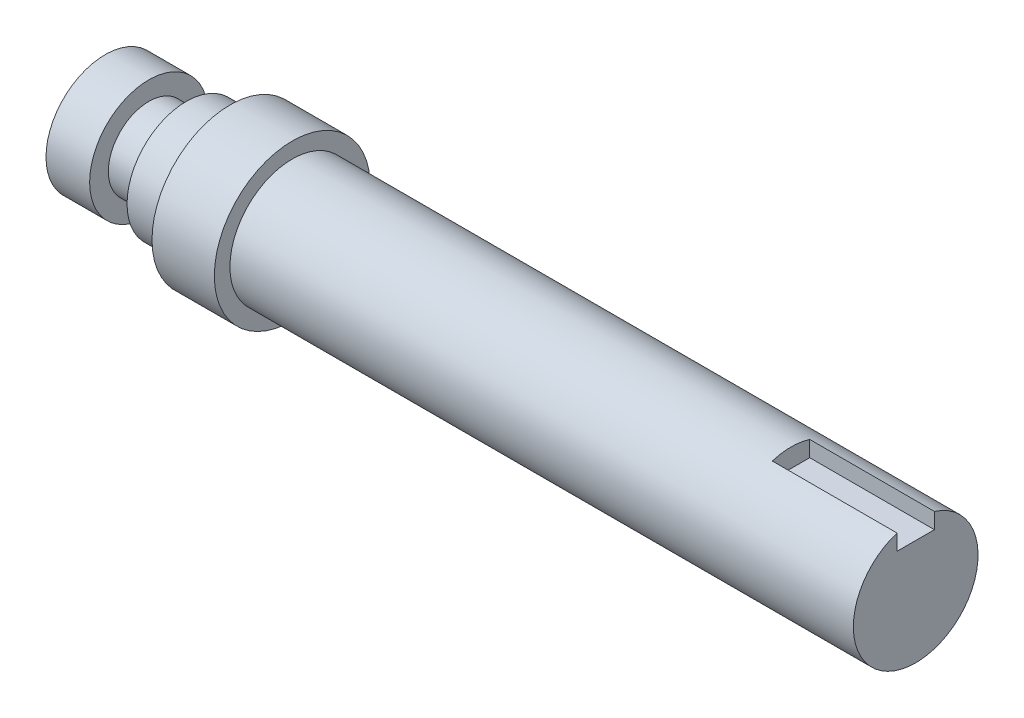
SolidWorks part; units mm, degrees
material "Plain Carbon Steel"
ref_plane "Front Plane" through (0, 0, 0) normal (0, 0, 1) x (1, 0, 0)
ref_plane "Top Plane" through (0, 0, 0) normal (0, 1, 0) x (1, 0, 0)
ref_plane "Right Plane" through (0, 0, 0) normal (1, 0, 0) x (0, 0, -1)
sketch "Shaft Profile Sketch" plane through (0, 0, 0) normal (0, 0, 1) x (1, 0, 0)
  line L0 (0, 0) -> (0, 9.5)
  line L1 (0, 9.5) -> (7, 9.5)
  line L2 (7, 9.5) -> (7, 6.5)
  line L3 (7, 6.5) -> (13, 6.5)
  line L4 (13, 6.5) -> (13, 9.5)
  line L5 (13, 9.5) -> (20, 9.5)
  line L6 (20, 9.5) -> (20, 12.5)
  line L7 (20, 12.5) -> (30, 12.5)
  line L8 (30, 12.5) -> (30, 10)
  line L9 (30, 10) -> (130, 10)
  line L10 (130, 10) -> (130, 0)
  line L11 (0, 0) -> (130, 0)
  dimension "D1" = 9.5
  dimension "D2" = 7
  dimension "D3" = 6
  dimension "D4" = 7
  dimension "D5" = 10
  dimension "D6" = 100
  dimension "D7" = 10
  dimension "D8" = 12.5
  dimension "D9" = 3
  dimension "D10" = 3
  dimension "D11" = 10
revolve "Stepped Shaft Body" add sketch "Shaft Profile Sketch" angle 360 about L11
sketch "Keyway Sketch" plane through (0, 0, 0) normal (0, 0, 1) x (1, 0, 0)
  line L1 (130, 7) -> (110, 7)
  line L2 (130, 7) -> (130, 12)
  line L3 (130, 12) -> (110, 12)
  line L4 (110, 7) -> (110, 12)
  line L5 (130, 7) -> (110, 12) construction
  line L6 (130, 12) -> (110, 7) construction
  line L8 (130, 10) -> (30, 10) construction
  point P0 (120, 9.5)
  dimension "D1" = 120
  dimension "D2" = 20
  dimension "D3" = 5
  dimension "D4" = 3
extrude "Keyway Cut" cut sketch "Keyway Sketch" against normal mid plane 6
